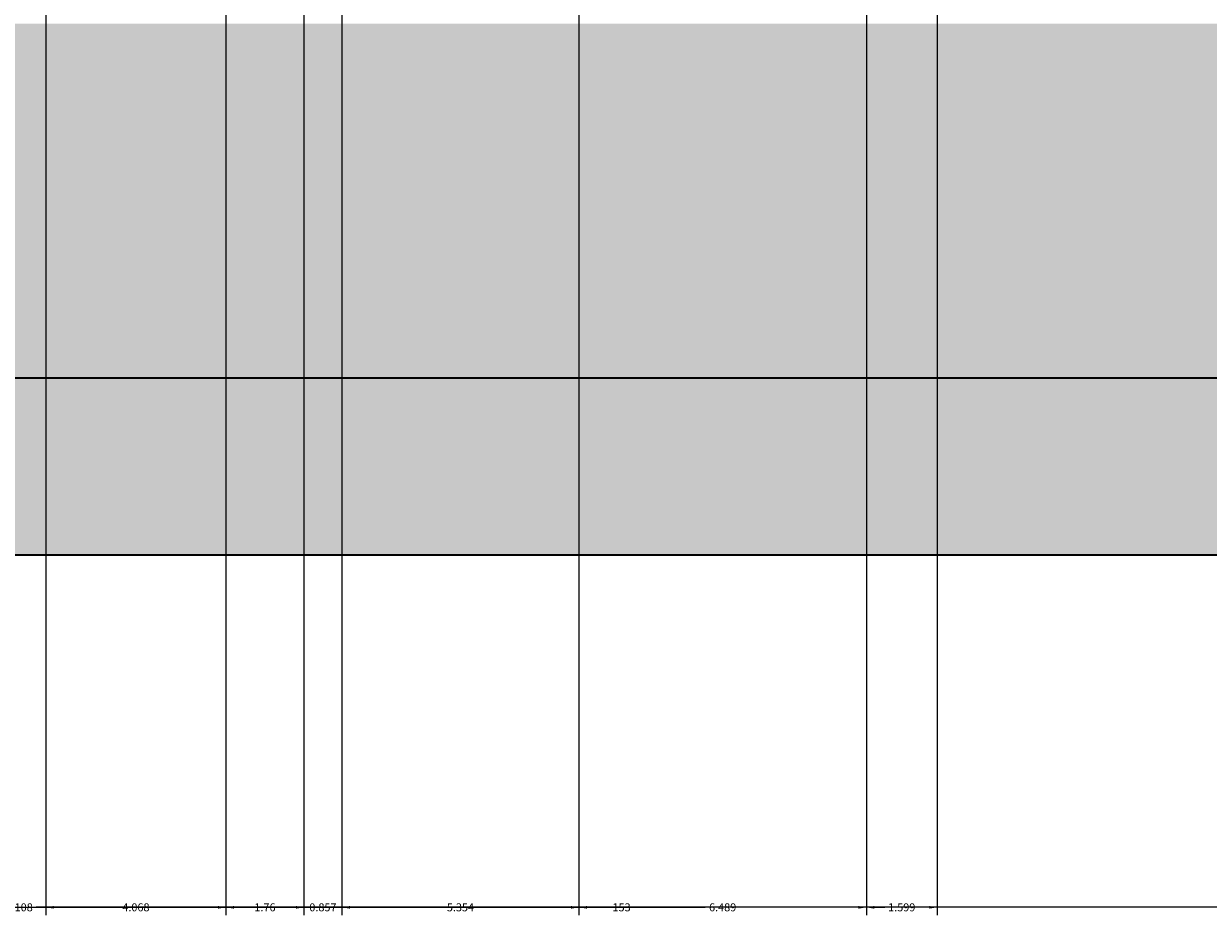
# Model space of a CAD drawing. Units: inches. Extents: x 4508 to 4723, y 847 to 1020.
# Tile 6 of 32: x 4604 to 4631, y 867 to 887. Entities that reach past the tile are written whole.
import ezdxf

# ---------------------------------------------------------------- set-up
doc = ezdxf.new("R2010")
doc.units = ezdxf.units.IN
for name, color, linetype, lineweight in [('A-ANNO-DIMS', 2, 'Continuous', 18), ('A-WALL', 7, 'Continuous', 35), ('A-WALL-PATT', 254, 'Continuous', 13)]:
    doc.layers.add(name, color=color, linetype=linetype, lineweight=lineweight)
doc.styles.get("Standard").update_dxf_attribs({"font": 'arial.ttf'})
doc.dimstyles.get("Standard").update_dxf_attribs({"dimtxt": 0.18, "dimasz": 0.18, "dimexe": 0.18, "dimexo": 0.0625, "dimgap": 0.09, "dimtad": 0, "dimtih": 1, "dimtoh": 1, "dimdec": 4, "dimzin": 0, "dimdsep": 46, "dimtxsty": 'Standard', "dimcen": 0.09, "dimadec": 0, "dimazin": 0, "dimtfac": 1, "dimtdec": 4, "dimtofl": 0, "dimtmove": 0, "dimatfit": 3, "dimfxl": 1, "dimtolj": 1, "dimtzin": 0, "dimarcsym": 0})

# ---------------------------------------------------------------- blocks, each defined once
blk = doc.blocks.new('*D2')
at = {"layer": 'A-ANNO-DIMS', "color": 0, "lineweight": -2, "transparency": 16777216}
for p, q in [((4540.994, 874.684), (4540.994, 866.617)), ((4693.994, 874.684), (4693.994, 866.617)), ((4541.174, 866.797), (4617.213, 866.797)), ((4693.814, 866.797), (4617.774, 866.797))]:
    blk.add_line(p, q, dxfattribs=at)
at = {"layer": 'A-ANNO-DIMS', "color": 0, "lineweight": 9, "transparency": 16777216}
for points in [[(4541.174, 866.827), (4541.174, 866.767), (4540.994, 866.797)], [(4693.814, 866.827), (4693.814, 866.767), (4693.994, 866.797)]]:
    blk.add_solid(points, dxfattribs=at)
at = {"layer": 'Defpoints', "color": 0, "lineweight": 9, "transparency": 16777216}
for p in [(4540.994, 874.747), (4693.994, 874.747), (4693.994, 866.797)]:
    blk.add_point(p, dxfattribs=at)
at = {"layer": 'A-ANNO-DIMS', "color": 0, "transparency": 16777216, "insert": (4617.494, 866.797), "char_height": 0.18, "attachment_point": 5}
blk.add_mtext('\\A1;153', dxfattribs=at)
blk = doc.blocks.new('*D24')
at = {"layer": 'A-ANNO-DIMS', "color": 0, "lineweight": -2, "transparency": 16777216}
for p, q in [((4549.994, 886.684), (4549.994, 866.617)), ((4657.994, 886.684), (4657.994, 866.617)), ((4550.174, 866.797), (4603.713, 866.797)), ((4657.814, 866.797), (4604.274, 866.797))]:
    blk.add_line(p, q, dxfattribs=at)
at = {"layer": 'A-ANNO-DIMS', "color": 0, "lineweight": 9, "transparency": 16777216}
for points in [[(4550.174, 866.827), (4550.174, 866.767), (4549.994, 866.797)], [(4657.814, 866.827), (4657.814, 866.767), (4657.994, 866.797)]]:
    blk.add_solid(points, dxfattribs=at)
at = {"layer": 'Defpoints', "color": 0, "lineweight": 9, "transparency": 16777216}
for p in [(4549.994, 886.747), (4657.994, 886.747), (4657.994, 866.797)]:
    blk.add_point(p, dxfattribs=at)
at = {"layer": 'A-ANNO-DIMS', "color": 0, "transparency": 16777216, "insert": (4603.994, 866.797), "char_height": 0.18, "attachment_point": 5}
blk.add_mtext('\\A1;108', dxfattribs=at)
blk = doc.blocks.new('*D33')
at = {"layer": 'A-ANNO-DIMS', "color": 0, "lineweight": -2, "transparency": 16777216}
for p, q in [((4604.494, 890.684), (4604.494, 866.617)), ((4608.562, 890.684), (4608.562, 866.617)), ((4604.674, 866.797), (4606.13, 866.797)), ((4608.382, 866.797), (4606.925, 866.797))]:
    blk.add_line(p, q, dxfattribs=at)
at = {"layer": 'A-ANNO-DIMS', "color": 0, "lineweight": 9, "transparency": 16777216}
for points in [[(4604.674, 866.827), (4604.674, 866.767), (4604.494, 866.797)], [(4608.382, 866.827), (4608.382, 866.767), (4608.562, 866.797)]]:
    blk.add_solid(points, dxfattribs=at)
at = {"layer": 'Defpoints', "color": 0, "lineweight": 9, "transparency": 16777216}
for p in [(4604.494, 890.747), (4608.562, 890.747), (4608.562, 866.797)]:
    blk.add_point(p, dxfattribs=at)
at = {"layer": 'A-ANNO-DIMS', "color": 0, "transparency": 16777216, "insert": (4606.528, 866.797), "char_height": 0.18, "attachment_point": 5}
blk.add_mtext('\\A1;4.068', dxfattribs=at)
blk = doc.blocks.new('*D36')
at = {"layer": 'A-ANNO-DIMS', "color": 0, "lineweight": -2, "transparency": 16777216}
for p, q in [((4610.322, 891.543), (4610.322, 866.617)), ((4608.562, 890.684), (4608.562, 866.617)), ((4608.742, 866.797), (4609.127, 866.797)), ((4610.142, 866.797), (4609.757, 866.797))]:
    blk.add_line(p, q, dxfattribs=at)
at = {"layer": 'A-ANNO-DIMS', "color": 0, "lineweight": 9, "transparency": 16777216}
for points in [[(4608.742, 866.827), (4608.742, 866.767), (4608.562, 866.797)], [(4610.142, 866.827), (4610.142, 866.767), (4610.322, 866.797)]]:
    blk.add_solid(points, dxfattribs=at)
at = {"layer": 'Defpoints', "color": 0, "lineweight": 9, "transparency": 16777216}
for p in [(4610.322, 891.605), (4608.562, 890.747), (4610.322, 866.797)]:
    blk.add_point(p, dxfattribs=at)
at = {"layer": 'A-ANNO-DIMS', "color": 0, "transparency": 16777216, "insert": (4609.442, 866.797), "char_height": 0.18, "attachment_point": 5}
blk.add_mtext('\\A1;1.76', dxfattribs=at)
blk = doc.blocks.new('*D37')
at = {"layer": 'A-ANNO-DIMS', "color": 0, "lineweight": -2, "transparency": 16777216}
for p, q in [((4610.322248, 891.542903), (4610.322248, 866.616874)), ((4611.179162, 891.534506), (4611.179162, 866.616874)), ((4610.142248, 866.796874), (4609.962248, 866.796874)), ((4611.359162, 866.796874), (4611.539162, 866.796874))]:
    blk.add_line(p, q, dxfattribs=at)
at = {"layer": 'A-ANNO-DIMS', "color": 0, "lineweight": 9, "transparency": 16777216}
for points in [[(4610.142248, 866.826874), (4610.142248, 866.766874), (4610.322248, 866.796874)], [(4611.359162, 866.826874), (4611.359162, 866.766874), (4611.179162, 866.796874)]]:
    blk.add_solid(points, dxfattribs=at)
at = {"layer": 'Defpoints', "color": 0, "lineweight": 9, "transparency": 16777216}
for p in [(4610.322248, 891.605403), (4611.179162, 891.597006), (4611.179162, 866.796874)]:
    blk.add_point(p, dxfattribs=at)
at = {"layer": 'A-ANNO-DIMS', "color": 0, "transparency": 16777216, "insert": (4610.750705, 866.796874), "char_height": 0.18, "attachment_point": 5}
blk.add_mtext('\\A1;0.857', dxfattribs=at)
blk = doc.blocks.new('*D38')
at = {"layer": 'A-ANNO-DIMS', "color": 0, "lineweight": -2, "transparency": 16777216}
for p, q in [((4616.533, 891.581), (4616.533, 866.617)), ((4611.179, 891.535), (4611.179, 866.617)), ((4611.359, 866.797), (4613.463, 866.797)), ((4616.353, 866.797), (4614.249, 866.797))]:
    blk.add_line(p, q, dxfattribs=at)
at = {"layer": 'A-ANNO-DIMS', "color": 0, "lineweight": 9, "transparency": 16777216}
for points in [[(4611.359, 866.827), (4611.359, 866.767), (4611.179, 866.797)], [(4616.353, 866.827), (4616.353, 866.767), (4616.533, 866.797)]]:
    blk.add_solid(points, dxfattribs=at)
at = {"layer": 'Defpoints', "color": 0, "lineweight": 9, "transparency": 16777216}
for p in [(4611.179, 891.597), (4616.533, 891.643), (4616.533, 866.797)]:
    blk.add_point(p, dxfattribs=at)
at = {"layer": 'A-ANNO-DIMS', "color": 0, "transparency": 16777216, "insert": (4613.856, 866.797), "char_height": 0.18, "attachment_point": 5}
blk.add_mtext('\\A1;5.354', dxfattribs=at)
blk = doc.blocks.new('*D39')
at = {"layer": 'A-ANNO-DIMS', "color": 0, "lineweight": -2, "transparency": 16777216}
for p, q in [((4616.533, 891.581), (4616.533, 866.617)), ((4623.022, 891.488), (4623.022, 866.617)), ((4616.713, 866.797), (4619.383, 866.797)), ((4622.842, 866.797), (4620.172, 866.797))]:
    blk.add_line(p, q, dxfattribs=at)
at = {"layer": 'A-ANNO-DIMS', "color": 0, "lineweight": 9, "transparency": 16777216}
for points in [[(4616.713, 866.827), (4616.713, 866.767), (4616.533, 866.797)], [(4622.842, 866.827), (4622.842, 866.767), (4623.022, 866.797)]]:
    blk.add_solid(points, dxfattribs=at)
at = {"layer": 'Defpoints', "color": 0, "lineweight": 9, "transparency": 16777216}
for p in [(4616.533, 891.643), (4623.022, 891.551), (4623.022, 866.797)]:
    blk.add_point(p, dxfattribs=at)
at = {"layer": 'A-ANNO-DIMS', "color": 0, "transparency": 16777216, "insert": (4619.777, 866.797), "char_height": 0.18, "attachment_point": 5}
blk.add_mtext('\\A1;6.489', dxfattribs=at)
blk = doc.blocks.new('*D40')
at = {"layer": 'A-ANNO-DIMS', "color": 0, "lineweight": -2, "transparency": 16777216}
for p, q in [((4623.022, 891.488), (4623.022, 866.617)), ((4624.621, 891.511), (4624.621, 866.617)), ((4623.202, 866.797), (4623.436, 866.797)), ((4624.441, 866.797), (4624.207, 866.797))]:
    blk.add_line(p, q, dxfattribs=at)
at = {"layer": 'A-ANNO-DIMS', "color": 0, "lineweight": 9, "transparency": 16777216}
for points in [[(4623.202, 866.827), (4623.202, 866.767), (4623.022, 866.797)], [(4624.441, 866.827), (4624.441, 866.767), (4624.621, 866.797)]]:
    blk.add_solid(points, dxfattribs=at)
at = {"layer": 'Defpoints', "color": 0, "lineweight": 9, "transparency": 16777216}
for p in [(4623.022, 891.551), (4624.621, 891.574), (4624.621, 866.797)]:
    blk.add_point(p, dxfattribs=at)
at = {"layer": 'A-ANNO-DIMS', "color": 0, "transparency": 16777216, "insert": (4623.821, 866.797), "char_height": 0.18, "attachment_point": 5}
blk.add_mtext('\\A1;1.599', dxfattribs=at)

msp = doc.modelspace()

# ---------------------------------------------------------------- hatches: boundary and pattern name
at = {"layer": 'A-WALL-PATT', "transparency": 33554508}
h = msp.add_hatch(color=256, dxfattribs=at)
h.dxf.hatch_style = 1
h.paths.add_polyline_path([(4661.6706, 954.043, -0.3739004), (4658.5765, 957.6021, -1), (4665.7646, 957.6021, -0.3739004), (4662.6706, 954.043), (4662.6706, 944.4021, -0.2114781), (4670.3062, 945.0869), (4670.3062, 968.0592, -0.4632086), (4663.3246, 973.9783, -0.4632086), (4670.3062, 979.8975), (4670.3062, 994.7469), (4588.9938, 994.7469), (4588.9938, 904.7469), (4657.9938, 904.7469), (4657.9938, 886.7469), (4549.9938, 886.7469), (4549.9938, 878.7469), (4693.9938, 878.7469), (4693.9938, 994.7469), (4671.8062, 994.7469), (4671.8062, 979.4411, -0.2941682), (4675.3246, 973.9783, -0.2941682), (4671.8062, 968.5156), (4671.8062, 944.4278, -0.2741114), (4676.7298, 936.1217, -0.2741114), (4671.8062, 927.8155), (4671.8062, 907.6998, -0.3779645), (4677.0562, 901.7469, -0.3779645), (4671.8062, 895.7939), (4671.8062, 883.7469), (4670.3062, 883.7469), (4670.3062, 895.7939, -0.3779645), (4665.0562, 901.7469, -0.3779645), (4670.3062, 907.6998), (4670.3062, 927.1564, -0.2114781), (4662.6706, 927.8412), (4662.6706, 918.2003, -0.3739004), (4665.7646, 914.6412, -1), (4658.5765, 914.6412, -0.3739004), (4661.6706, 918.2003), (4661.6706, 928.4807, -0.2391825), (4657.7936, 936.1217, -0.2391825), (4661.6706, 943.7626)])
at = {"layer": 'A-WALL-PATT', "transparency": 33554556}
h = msp.add_hatch(color=256, dxfattribs=at)
h.dxf.hatch_style = 1
h.paths.add_polyline_path([(4689.9938, 878.7469), (4549.9938, 878.7469), (4549.9938, 874.7469), (4689.9938, 874.7469)])

# ---------------------------------------------------------------- linework, layer by layer
at = {"layer": 'A-WALL'}
for p, q in [((4693.9938, 878.7469), (4549.9938, 878.7469)), ((4693.9938, 874.7469), (4549.9938, 874.7469))]:
    msp.add_line(p, q, dxfattribs=at)

# ---------------------------------------------------------------- dimensions: what is measured, and where the dimension line sits
at = {"layer": 'A-ANNO-DIMS'}
for base, p1, p2, override, picture, middle in [((4610.3222, 866.7969), (4608.5617, 890.7469), (4610.3222, 891.6054), {"dimdec": 2, "dimlfac": 1, "dimrnd": 0, "dimzin": 0, "dimdsep": 46, "dimlunit": 2}, '*D36', (4609.442, 866.7969)), ((4611.1792, 866.7969), (4610.3222, 891.6054), (4611.1792, 891.597), {"dimdec": 3, "dimlfac": 1, "dimrnd": 0, "dimzin": 0, "dimdsep": 46, "dimlunit": 2}, '*D37', (4610.7507, 866.7969)), ((4616.5328, 866.7969), (4611.1792, 891.597), (4616.5328, 891.6433), {"dimdec": 3, "dimlfac": 1, "dimrnd": 0, "dimzin": 0, "dimdsep": 46, "dimlunit": 2}, '*D38', (4613.856, 866.7969)), ((4623.0217, 866.7969), (4616.5328, 891.6433), (4623.0217, 891.5507), {"dimdec": 3, "dimlfac": 1, "dimrnd": 0, "dimzin": 0, "dimdsep": 46, "dimlunit": 2}, '*D39', (4619.7773, 866.7969)), ((4624.6207, 866.7969), (4623.0217, 891.5507), (4624.6207, 891.5739), {"dimdec": 3, "dimlfac": 1, "dimrnd": 0, "dimzin": 0, "dimdsep": 46, "dimlunit": 2}, '*D40', (4623.8212, 866.7969)), ((4608.5617, 866.7969), (4604.4938, 890.7469), (4608.5617, 890.7469), {"dimdec": 3, "dimlfac": 1, "dimrnd": 0, "dimzin": 0, "dimdsep": 46, "dimlunit": 2}, '*D33', (4606.5277, 866.7969)), ((4657.9938, 866.7969), (4549.9938, 886.7469), (4657.9938, 886.7469), {"dimdec": 0, "dimlfac": 1, "dimrnd": 0, "dimzin": 0, "dimdsep": 46, "dimlunit": 2}, '*D24', (4603.9938, 866.7969)), ((4693.9938, 866.7969), (4540.9938, 874.7469), (4693.9938, 874.7469), {"dimdec": 0, "dimlfac": 1, "dimrnd": 0, "dimzin": 0, "dimdsep": 46, "dimlunit": 2}, '*D2', (4617.4938, 866.7969))]:
    dim = msp.add_linear_dim(base=base, p1=p1, p2=p2, dimstyle='Standard', override=override, dxfattribs=at)
    dim.commit()
    dim.dimension.update_dxf_attribs({"geometry": picture, "text_midpoint": middle})

doc.saveas('drawing.dxf')
